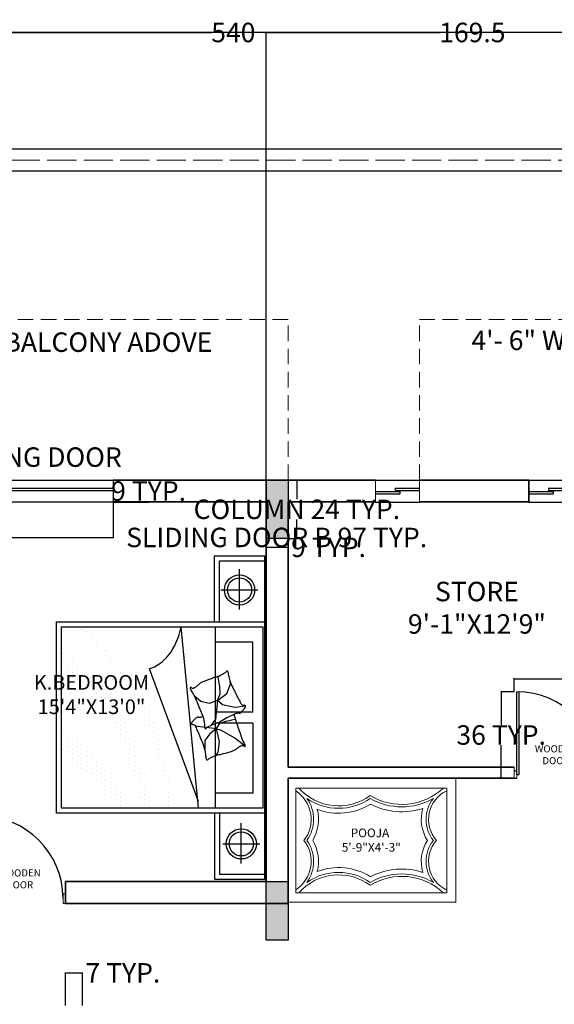
# Model space of a CAD drawing. Units: inches. Extents: x -48 to 50072, y 0 to 21068.
# Tile 55 of 75: x 196 to 415, y 819 to 1224. Entities that reach past the tile are written whole.
import ezdxf

# ---------------------------------------------------------------- set-up
doc = ezdxf.new("R2010")
doc.units = ezdxf.units.IN
doc.header["$MEASUREMENT"] = 0
doc.linetypes.add('ACAD_ISO02W100', pattern=[15, 12, -3])
doc.linetypes.add('HIDDEN', pattern=[9.525, 6.35, -3.175])
for name, color, linetype, lineweight in [('A-ANNO-DIMS', 2, 'Continuous', 18), ('A-ANNO-TEXT', 7, 'Continuous', 18), ('A-AREA-IDEN', 7, 'Continuous', 18), ('A-COLS', 1, 'Continuous', 35), ('A-DOOR', 4, 'Continuous', 18), ('A-FLOR-CASE', 9, 'Continuous', 18), ('A-FLOR-OVHD', 8, 'HIDDEN', 13), ('A-GLAZ', 4, 'Continuous', 18), ('A-WALL', 7, 'Continuous', 35), ('C-PROP', 7, 'Continuous', 25), ('C-PROP-REF', 32, 'ACAD_ISO02W100', 13), ('FURNITURE', 44, 'Continuous', 18)]:
    doc.layers.add(name, color=color, linetype=linetype, lineweight=lineweight)
doc.layers.add('Layer3', color=176, linetype='Continuous')
doc.styles.get("Standard").update_dxf_attribs({"font": 'arial.ttf'})
doc.dimstyles.get("Standard").update_dxf_attribs({"dimtxt": 8, "dimasz": 0.18, "dimexe": 0.18, "dimexo": 0.0625, "dimgap": 0.09, "dimtad": 0, "dimtih": 1, "dimtoh": 1, "dimdec": 1, "dimzin": 0, "dimdsep": 46, "dimlunit": 4, "dimtxsty": 'Standard', "dimblk": 'ARCHTICK', "dimcen": 0.09, "dimadec": 0, "dimazin": 0, "dimtfac": 1, "dimtdec": 1, "dimtofl": 0, "dimtmove": 0, "dimatfit": 3, "dimldrblk": 'ARCHTICK', "dimfxl": 1, "dimtolj": 1, "dimtzin": 0, "dimarcsym": 0})

# ---------------------------------------------------------------- blocks, each defined once
blk = doc.blocks.new('BKUHJKKUG')
at = {"layer": 'Defpoints'}
for p, q in [((179.52, 862.77), (179.52, 896.77)), ((180.52, 862.77), (180.52, 896.76)), ((179.52, 862.77), (180.52, 862.77))]:
    blk.add_line(p, q, dxfattribs=at)
blk.add_arc((179.52, 862.77), 34, 0, 90, dxfattribs=at)
at = {"insert": (190.84, 874.8), "char_height": 2.9183, "attachment_point": 1}
blk.add_mtext_dynamic_manual_height_columns('\\pxqc;WOODEN ^JDOOR', width=9.6242, gutter_width=14.59, heights=[0], dxfattribs=at)
blk = doc.blocks.new('sliding')
blk.add_line((137.02, 1025.77), (137.02, 1034.77))
at = {"layer": 'Defpoints'}
for p, q in [((234.12, 1034.77), (234.12, 1025.77)), ((137.02, 1030.07), (187.57, 1030.07)), ((137.02, 1029.07), (187.57, 1029.07)), ((183.57, 1031.47), (234.12, 1031.47)), ((183.57, 1031.47), (183.57, 1030.47)), ((183.57, 1030.47), (234.12, 1030.47)), ((187.57, 1030.07), (187.57, 1029.07))]:
    blk.add_line(p, q, dxfattribs=at)
at = {"layer": 'Layer3'}
for p, q in [((137.02, 1034.77), (234.12, 1034.77)), ((234.12, 1025.77), (137.02, 1025.77))]:
    blk.add_line(p, q, dxfattribs=at)
blk = doc.blocks.new('bnniku')
at = {"layer": 'Defpoints'}
h = blk.add_hatch(color=256, dxfattribs=at)
h.dxf.hatch_style = 1
h.paths.add_polyline_path([(767.55, 1114.04), (758.55, 1114.04), (758.55, 1090.04), (767.55, 1090.04)])
for p, q in [((758.55, 1114.04), (767.55, 1114.04)), ((758.55, 1090.04), (758.55, 1114.04)), ((767.55, 1114.04), (767.55, 1090.04)), ((767.55, 1090.04), (758.55, 1090.04))]:
    blk.add_line(p, q, dxfattribs=at)
blk = doc.blocks.new('jyugcli')
for p, q in [((342.02, 1025.77), (342.02, 1034.77)), ((360.02, 1025.77), (360.02, 1034.77))]:
    blk.add_line(p, q)
at = {"layer": 'Defpoints'}
for p, q in [((342.02, 1030.07), (352.02, 1030.07)), ((342.02, 1029.07), (352.02, 1029.07)), ((350.02, 1031.47), (360.02, 1031.47)), ((350.02, 1031.47), (350.02, 1030.47)), ((350.02, 1030.47), (360.02, 1030.47)), ((352.02, 1030.07), (352.02, 1029.07))]:
    blk.add_line(p, q, dxfattribs=at)
at = {"layer": 'Layer3'}
for p, q in [((342.02, 1034.77), (360.02, 1034.77)), ((342.02, 1025.77), (360.02, 1025.77))]:
    blk.add_line(p, q, dxfattribs=at)
blk = doc.blocks.new('yfhjudru')
for p, q in [((399.02, 912.27), (399.02, 916.77)), ((400.02, 912.27), (400.02, 915.27)), ((434.02, 912.27), (434.02, 915.27)), ((435.02, 912.27), (435.02, 916.77))]:
    blk.add_line(p, q)
at = {"layer": 'Defpoints'}
for p, q in [((399.02, 915.27), (400.02, 915.27)), ((434.02, 915.27), (435.02, 915.27)), ((399.02, 912.27), (400.02, 912.27)), ((434.02, 912.27), (435.02, 912.27))]:
    blk.add_line(p, q, dxfattribs=at)
blk.add_blockref('BKUHJKKUG', (220.5, 51), dxfattribs=at)
blk = doc.blocks.new('nhrygfdu7yu')
at = {"layer": 'Defpoints'}
for p, q in [((1019.17, 828.61), (845.97, 828.61)), ((845.97, 801.61), (845.97, 828.61)), ((848.67, 804.31), (848.67, 828.61)), ((881.27, 716.83), (881.27, 828.61)), ((983.87, 828.61), (983.87, 716.83)), ((1016.47, 804.31), (1016.47, 828.61)), ((1019.17, 801.61), (1019.17, 828.61)), ((864.18, 805.04), (864.18, 824.84)), ((884.03, 719.53), (884.03, 827.53)), ((884.03, 827.53), (981.17, 827.53)), ((981.17, 827.53), (981.17, 719.53)), ((1000.24, 805.98), (1000.24, 825.78)), ((892.12, 822.13), (892.12, 801.97)), ((929.67, 822.13), (892.12, 822.13)), ((926.47, 818.07), (927.21, 812.5)), ((929.67, 822.13), (929.67, 801.78)), ((935.52, 822.13), (935.52, 801.78)), ((935.52, 822.13), (973.07, 822.13)), ((947.88, 818.06), (943.61, 812.45)), ((973.07, 822.13), (973.07, 801.97)), ((874.65, 814.99), (853.09, 814.99)), ((927.21, 812.5), (925.82, 805.91)), ((934.43, 807.75), (933.36, 812.55)), ((1010.72, 815.93), (989.15, 815.93)), ((914.58, 810.18), (913.28, 809.99)), ((919.69, 808.14), (914.58, 810.18)), ((923.4, 803.12), (919.69, 808.14)), ((935.49, 804.66), (934.43, 807.75)), ((943.61, 812.45), (939.55, 805.41)), ((881.07, 804.31), (848.67, 804.31)), ((881.07, 804.31), (881.07, 804.31)), ((884.06, 801.97), (981.18, 801.97)), ((910.77, 803.49), (910.59, 803.15)), ((916.07, 804.42), (910.77, 803.49)), ((919.78, 804.61), (916.07, 804.42)), ((923.4, 803.12), (919.78, 804.61)), ((925.82, 805.91), (923.4, 803.12)), ((923.4, 803.12), (925.08, 798.67)), ((923.4, 803.12), (933.44, 802.1)), ((933.44, 802.1), (936.13, 800.15)), ((935.45, 803.17), (936.69, 800.13)), ((938.59, 802.42), (935.49, 804.66)), ((938.59, 802.42), (937.95, 797.34)), ((939.55, 805.41), (938.59, 802.42)), ((938.59, 802.42), (945.53, 804.13)), ((938.59, 802.42), (941.26, 799.01)), ((945.53, 804.13), (951.08, 803.38)), ((951.08, 803.38), (953.02, 802.3)), ((984.07, 804.31), (1016.47, 804.31)), ((984.07, 804.31), (984.07, 804.31)), ((881.07, 801.61), (845.97, 801.61)), ((925.08, 798.67), (923.96, 794.21)), ((936.13, 800.15), (936.78, 799.69)), ((936.69, 800.13), (937.65, 797.78)), ((941.26, 799.01), (944.78, 796.45)), ((984.07, 801.61), (1019.17, 801.61)), ((981.13, 793.06), (883.98, 783.7)), ((906.36, 766.47), (977.44, 792.73)), ((923.96, 794.21), (921.07, 790.83)), ((937.86, 796.54), (937.22, 791.44)), ((944.78, 796.45), (949.8, 796.45)), ((962.27, 776.79), (962.27, 776.79)), ((964.84, 776.79), (964.84, 776.79)), ((967.41, 776.79), (967.41, 776.79)), ((969.98, 776.79), (969.98, 776.79)), ((972.55, 776.79), (972.55, 776.79)), ((975.13, 776.79), (975.13, 776.79)), ((976.41, 779.36), (976.41, 779.36)), ((977.7, 776.79), (977.7, 776.79)), ((978.98, 779.36), (978.98, 779.36)), ((980.27, 776.79), (980.27, 776.79)), ((941.69, 771.64), (941.69, 771.64)), ((944.27, 771.64), (944.27, 771.64)), ((946.84, 771.64), (946.84, 771.64)), ((949.41, 771.64), (949.41, 771.64)), ((950.69, 774.21), (950.69, 774.21)), ((951.98, 771.64), (951.98, 771.64)), ((953.27, 774.21), (953.27, 774.21)), ((954.55, 771.64), (954.55, 771.64)), ((955.84, 774.21), (955.84, 774.21)), ((958.41, 774.21), (958.41, 774.21)), ((960.98, 774.21), (960.98, 774.21)), ((963.55, 774.21), (963.55, 774.21)), ((966.13, 774.21), (966.13, 774.21)), ((968.7, 774.21), (968.7, 774.21)), ((928.83, 766.5), (928.83, 766.5)), ((931.41, 766.5), (931.41, 766.5)), ((933.98, 766.5), (933.98, 766.5)), ((935.26, 769.07), (935.26, 769.07)), ((936.55, 766.5), (936.55, 766.5)), ((937.84, 769.07), (937.84, 769.07)), ((940.41, 769.07), (940.41, 769.07)), ((942.98, 769.07), (942.98, 769.07)), ((975.13, 766.5), (975.13, 766.5)), ((977.7, 766.5), (977.7, 766.5)), ((980.27, 766.5), (980.27, 766.5)), ((921.12, 761.35), (921.12, 761.35)), ((923.69, 761.35), (923.69, 761.35)), ((924.98, 763.93), (924.98, 763.93)), ((927.55, 763.93), (927.55, 763.93)), ((930.12, 763.93), (930.12, 763.93)), ((954.55, 761.35), (954.55, 761.35)), ((957.12, 761.35), (957.12, 761.35)), ((959.7, 761.35), (959.7, 761.35)), ((962.27, 761.35), (962.27, 761.35)), ((963.55, 763.93), (963.55, 763.93)), ((964.84, 761.35), (964.84, 761.35)), ((966.13, 763.93), (966.13, 763.93)), ((967.41, 761.35), (967.41, 761.35)), ((968.7, 763.93), (968.7, 763.93)), ((969.98, 761.35), (969.98, 761.35)), ((971.27, 763.93), (971.27, 763.93)), ((972.55, 761.35), (972.55, 761.35)), ((973.84, 763.93), (973.84, 763.93)), ((975.13, 761.35), (975.13, 761.35)), ((976.41, 763.93), (976.41, 763.93)), ((978.98, 763.93), (978.98, 763.93)), ((913.4, 756.21), (913.4, 756.21)), ((915.98, 756.21), (915.98, 756.21)), ((917.26, 758.78), (917.26, 758.78)), ((919.83, 758.78), (919.83, 758.78)), ((941.69, 756.21), (941.69, 756.21)), ((944.27, 756.21), (944.27, 756.21)), ((945.55, 758.78), (945.55, 758.78)), ((946.84, 756.21), (946.84, 756.21)), ((948.12, 758.78), (948.12, 758.78)), ((949.41, 756.21), (949.41, 756.21)), ((950.69, 758.78), (950.69, 758.78)), ((951.98, 756.21), (951.98, 756.21)), ((953.27, 758.78), (953.27, 758.78)), ((954.55, 756.21), (954.55, 756.21)), ((955.84, 758.78), (955.84, 758.78)), ((957.12, 756.21), (957.12, 756.21)), ((958.41, 758.78), (958.41, 758.78)), ((960.98, 758.78), (960.98, 758.78)), ((963.55, 758.78), (963.55, 758.78)), ((980.27, 756.21), (980.27, 756.21)), ((905.69, 751.07), (905.69, 751.07)), ((908.26, 751.07), (908.26, 751.07)), ((909.55, 753.64), (909.55, 753.64)), ((912.12, 753.64), (912.12, 753.64)), ((931.41, 751.07), (931.41, 751.07)), ((933.98, 751.07), (933.98, 751.07)), ((935.26, 753.64), (935.26, 753.64)), ((936.55, 751.07), (936.55, 751.07)), ((937.84, 753.64), (937.84, 753.64)), ((939.12, 751.07), (939.12, 751.07)), ((940.41, 753.64), (940.41, 753.64)), ((941.69, 751.07), (941.69, 751.07)), ((942.98, 753.64), (942.98, 753.64)), ((944.27, 751.07), (944.27, 751.07)), ((945.55, 753.64), (945.55, 753.64)), ((948.12, 753.64), (948.12, 753.64)), ((969.98, 751.07), (969.98, 751.07)), ((972.55, 751.07), (972.55, 751.07)), ((975.13, 751.07), (975.13, 751.07)), ((976.41, 753.64), (976.41, 753.64)), ((977.7, 751.07), (977.7, 751.07)), ((978.98, 753.64), (978.98, 753.64)), ((980.27, 751.07), (980.27, 751.07)), ((900.55, 745.92), (900.55, 745.92)), ((903.12, 745.92), (903.12, 745.92)), ((904.4, 748.5), (904.4, 748.5)), ((923.69, 745.92), (923.69, 745.92)), ((926.26, 745.92), (926.26, 745.92)), ((927.55, 748.5), (927.55, 748.5)), ((928.83, 745.92), (928.83, 745.92)), ((930.12, 748.5), (930.12, 748.5)), ((931.41, 745.92), (931.41, 745.92)), ((932.69, 748.5), (932.69, 748.5)), ((933.98, 745.92), (933.98, 745.92)), ((935.26, 748.5), (935.26, 748.5)), ((937.84, 748.5), (937.84, 748.5)), ((940.41, 748.5), (940.41, 748.5)), ((962.27, 745.92), (962.27, 745.92)), ((964.84, 745.92), (964.84, 745.92)), ((966.13, 748.5), (966.13, 748.5)), ((967.41, 745.92), (967.41, 745.92)), ((968.7, 748.5), (968.7, 748.5)), ((969.98, 745.92), (969.98, 745.92)), ((971.27, 748.5), (971.27, 748.5)), ((972.55, 745.92), (972.55, 745.92)), ((973.84, 748.5), (973.84, 748.5)), ((975.13, 745.92), (975.13, 745.92)), ((976.41, 748.5), (976.41, 748.5)), ((977.7, 745.92), (977.7, 745.92)), ((978.98, 748.5), (978.98, 748.5)), ((895.4, 740.78), (895.4, 740.78)), ((896.69, 743.35), (896.69, 743.35)), ((899.26, 743.35), (899.26, 743.35)), ((915.98, 740.78), (915.98, 740.78)), ((918.55, 740.78), (918.55, 740.78)), ((919.83, 743.35), (919.83, 743.35)), ((921.12, 740.78), (921.12, 740.78)), ((922.41, 743.35), (922.41, 743.35)), ((923.69, 740.78), (923.69, 740.78)), ((924.98, 743.35), (924.98, 743.35)), ((926.26, 740.78), (926.26, 740.78)), ((927.55, 743.35), (927.55, 743.35)), ((928.83, 740.78), (928.83, 740.78)), ((930.12, 743.35), (930.12, 743.35)), ((932.69, 743.35), (932.69, 743.35)), ((957.12, 740.78), (957.12, 740.78)), ((959.7, 740.78), (959.7, 740.78)), ((960.98, 743.35), (960.98, 743.35)), ((962.27, 740.78), (962.27, 740.78)), ((963.55, 743.35), (963.55, 743.35)), ((964.84, 740.78), (964.84, 740.78)), ((966.13, 743.35), (966.13, 743.35)), ((967.41, 740.78), (967.41, 740.78)), ((968.7, 743.35), (968.7, 743.35)), ((969.98, 740.78), (969.98, 740.78)), ((971.27, 743.35), (971.27, 743.35)), ((973.84, 743.35), (973.84, 743.35)), ((887.69, 735.64), (887.69, 735.64)), ((890.26, 735.64), (890.26, 735.64)), ((891.54, 738.21), (891.54, 738.21)), ((894.12, 738.21), (894.12, 738.21)), ((910.83, 735.64), (910.83, 735.64)), ((913.4, 735.64), (913.4, 735.64)), ((914.69, 738.21), (914.69, 738.21)), ((915.98, 735.64), (915.98, 735.64)), ((917.26, 738.21), (917.26, 738.21)), ((918.55, 735.64), (918.55, 735.64)), ((919.83, 738.21), (919.83, 738.21)), ((921.12, 735.64), (921.12, 735.64)), ((922.41, 738.21), (922.41, 738.21)), ((924.98, 738.21), (924.98, 738.21)), ((951.98, 735.64), (951.98, 735.64)), ((954.55, 735.64), (954.55, 735.64)), ((955.84, 738.21), (955.84, 738.21)), ((957.12, 735.64), (957.12, 735.64)), ((958.41, 738.21), (958.41, 738.21)), ((959.7, 735.64), (959.7, 735.64)), ((960.98, 738.21), (960.98, 738.21)), ((962.27, 735.64), (962.27, 735.64)), ((963.55, 738.21), (963.55, 738.21)), ((964.84, 735.64), (964.84, 735.64)), ((966.13, 738.21), (966.13, 738.21)), ((885.12, 730.49), (885.12, 730.49)), ((886.4, 733.07), (886.4, 733.07)), ((888.97, 733.07), (888.97, 733.07)), ((905.69, 730.49), (905.69, 730.49)), ((908.26, 730.49), (908.26, 730.49)), ((909.55, 733.07), (909.55, 733.07)), ((910.83, 730.49), (910.83, 730.49)), ((912.12, 733.07), (912.12, 733.07)), ((913.4, 730.49), (913.4, 730.49)), ((914.69, 733.07), (914.69, 733.07)), ((915.98, 730.49), (915.98, 730.49)), ((917.26, 733.07), (917.26, 733.07)), ((919.83, 733.07), (919.83, 733.07)), ((946.84, 730.49), (946.84, 730.49)), ((949.41, 730.49), (949.41, 730.49)), ((950.69, 733.07), (950.69, 733.07)), ((951.98, 730.49), (951.98, 730.49)), ((953.27, 733.07), (953.27, 733.07)), ((954.55, 730.49), (954.55, 730.49)), ((955.84, 733.07), (955.84, 733.07)), ((957.12, 730.49), (957.12, 730.49)), ((958.41, 733.07), (958.41, 733.07)), ((959.7, 730.49), (959.7, 730.49)), ((960.98, 733.07), (960.98, 733.07)), ((900.55, 725.35), (900.55, 725.35)), ((903.12, 725.35), (903.12, 725.35)), ((904.4, 727.92), (904.4, 727.92)), ((905.69, 725.35), (905.69, 725.35)), ((906.97, 727.92), (906.97, 727.92)), ((908.26, 725.35), (908.26, 725.35)), ((909.55, 727.92), (909.55, 727.92)), ((910.83, 725.35), (910.83, 725.35)), ((912.12, 727.92), (912.12, 727.92)), ((944.27, 725.35), (944.27, 725.35)), ((945.55, 727.92), (945.55, 727.92)), ((946.84, 725.35), (946.84, 725.35)), ((948.12, 727.92), (948.12, 727.92)), ((949.41, 725.35), (949.41, 725.35)), ((950.69, 727.92), (950.69, 727.92)), ((951.98, 725.35), (951.98, 725.35)), ((953.27, 727.92), (953.27, 727.92)), ((954.55, 725.35), (954.55, 725.35)), ((955.84, 727.92), (955.84, 727.92)), ((958.41, 727.92), (958.41, 727.92)), ((981.17, 719.53), (884.03, 719.53)), ((895.4, 720.21), (895.4, 720.21)), ((897.97, 720.21), (897.97, 720.21)), ((899.26, 722.78), (899.26, 722.78)), ((900.55, 720.21), (900.55, 720.21)), ((901.83, 722.78), (901.83, 722.78)), ((903.12, 720.21), (903.12, 720.21)), ((904.4, 722.78), (904.4, 722.78)), ((905.69, 720.21), (905.69, 720.21)), ((906.97, 722.78), (906.97, 722.78)), ((939.12, 720.21), (939.12, 720.21)), ((941.69, 720.21), (941.69, 720.21)), ((942.98, 722.78), (942.98, 722.78)), ((944.27, 720.21), (944.27, 720.21)), ((945.55, 722.78), (945.55, 722.78)), ((946.84, 720.21), (946.84, 720.21)), ((948.12, 722.78), (948.12, 722.78)), ((949.41, 720.21), (949.41, 720.21)), ((950.69, 722.78), (950.69, 722.78)), ((951.98, 720.21), (951.98, 720.21)), ((953.27, 722.78), (953.27, 722.78)), ((983.87, 716.83), (881.27, 716.83))]:
    blk.add_line(p, q, dxfattribs=at)
for centre, radius in [((864.18, 814.99), 8.1), ((1000.24, 815.93), 8.1), ((864.18, 814.99), 6.48), ((1000.24, 815.93), 6.48)]:
    blk.add_circle(centre, radius, dxfattribs=at)
for centre, radius, start, end in [((926.67, 817.58), 0.687, 51.1864, 183.2455), ((924.75, 815.18), 3.76, 45.8726, 51.1864), ((929.07, 819.63), 2.44, 225.8726, 232.4713), ((948.22, 814.9), 3.25, 110.3452, 128.5854), ((947.75, 816.16), 1.9, 86.0516, 110.3452), ((947.87, 817.82), 0.239, 13.2808, 86.0516), ((947.77, 817.8), 0.34, 306.5792, 13.2808), ((771.78, 1091.44), 315.27, 297.4921, 297.8482), ((1072.97, 521.35), 329.5, 117.4999, 117.8482), ((971.1, 717.04), 108.88, 116.4147, 117.4999), ((848.26, 964.34), 167.25, 296.4147, 297.2902), ((924.05, 817.43), 1.94, 297.2902, 3.2455), ((940.16, 834.08), 20.66, 232.4713, 233.7837), ((906.88, 788.64), 35.67, 52.7849, 53.7837), ((921.35, 807.68), 11.75, 46.4776, 52.7849), ((926.56, 813.17), 4.18, 35.8936, 46.4776), ((928.96, 814.91), 1.22, 351.9508, 35.8936), ((932.62, 814.39), 2.47, 171.9508, 202.4162), ((980.52, 834.15), 54.29, 202.4162, 205.0529), ((883.03, 974.91), 169.83, 286.6085, 289.0836), ((848.62, 1074.38), 275.09, 289.0836, 290.1287), ((927.73, 858.54), 45.2, 290.1287, 292.7069), ((943.53, 820.78), 4.28, 292.7069, 308.5854), ((951.77, 816.3), 4.17, 169.5926, 177.2714), ((948.44, 816.46), 0.826, 177.2714, 194.5709), ((949.69, 816.78), 2.12, 194.5709, 206.8179), ((948.43, 816.91), 0.765, 126.5792, 169.5926), ((964.76, 824.4), 19.01, 206.8179, 210.9056), ((957.44, 820.02), 10.47, 210.9056, 219.7005), ((946.01, 810.53), 4.37, 26.0735, 39.7005), ((908.02, 808.45), 0.313, 121.6917, 179.0386), ((908.61, 808.44), 0.905, 179.0386, 229.4914), ((909.3, 806.38), 2.75, 103.0402, 121.6917), ((905.38, 804.66), 4.08, 26.3332, 49.4914), ((909.41, 805.91), 3.23, 86.6119, 103.0402), ((909.8, 812.53), 3.4, 266.6119, 282.6252), ((905.47, 831.87), 23.22, 282.6252, 290.7486), ((901.77, 841.65), 33.68, 290.7486, 297.4921), ((929.77, 818.2), 6.29, 280.7366, 286.6085), ((1013.86, 849.73), 91.09, 205.0529, 207.0884), ((1008.01, 846.74), 84.52, 207.0884, 209.936), ((940.41, 807.79), 10.61, 17.8396, 26.0735), ((847.55, 777.91), 108.16, 15.2625, 17.8396), ((780.21, 742.7), 143.74, 25.1732, 26.3332), ((901.51, 799.71), 9.71, 20.7081, 25.1732), ((883.04, 792.73), 29.45, 18.2369, 20.7081), ((995.54, 829.8), 89, 198.2369, 199.6584), ((924.73, 798.79), 11.57, 22.2355, 29.936), ((866.04, 782.95), 89, 13.841, 15.2625), ((981.05, 811.29), 29.45, 193.841, 196.3122), ((962.1, 805.74), 9.71, 196.3122, 200.7773), ((1087.42, 853.29), 143.74, 200.7773, 201.9373), ((1013.59, 836.25), 108.16, 199.6584, 202.2355), ((938.8, 798.25), 1.24, 202.2355, 252.8133), ((938.36, 796.82), 0.252, 289.3799, 72.8133), ((955.69, 773.98), 23.22, 98.2293, 106.3527), ((952.85, 793.6), 3.4, 82.216, 98.2293), ((953.75, 800.17), 3.23, 262.216, 278.6443), ((957.87, 801.11), 4.08, 201.9373, 225.0955), ((953.82, 799.69), 2.75, 278.6443, 297.2959), ((954.35, 797.58), 0.905, 354.6428, 45.0955), ((954.94, 797.53), 0.313, 297.2959, 354.6428), ((923.29, 799.33), 10.61, 202.2355, 210.4694), ((917.92, 796.17), 4.37, 210.4694, 224.0964), ((907.26, 785.84), 10.47, 35.3015, 44.0964), ((900.29, 780.91), 19.01, 31.2138, 35.3015), ((1035.25, 540.56), 275.09, 113.4795, 114.5246), ((993.31, 637.11), 169.83, 111.0043, 113.4795), ((880.68, 777.46), 54.29, 18.0203, 19.3448), ((929.96, 793.49), 2.47, 347.5549, 18.0203), ((933.57, 792.7), 1.22, 167.5549, 211.4977), ((934.7, 789.77), 6.29, 98.1216, 111.0043), ((936.09, 794.24), 4.18, 211.4977, 222.0817), ((941.71, 799.32), 11.75, 222.0817, 228.389), ((934.31, 792.46), 3.58, 85.4882, 98.1216), ((934.9, 799.87), 3.85, 265.4882, 277.6784), ((934.12, 805.65), 9.69, 277.6784, 284.8807), ((938.27, 789.81), 1.94, 112.8944, 178.8496), ((939.32, 786.09), 10.56, 97.9822, 104.8807), ((1002.58, 637.52), 167.25, 112.0188, 112.8944), ((938.1, 794.73), 1.83, 85.7407, 97.9822), ((938.28, 797.05), 0.497, 265.7407, 289.3799), ((899.06, 893.51), 108.88, 292.0188, 293.104), ((812.48, 1096.43), 329.5, 293.104, 293.4523), ((1069.09, 504.93), 315.27, 113.0962, 113.4523), ((958.63, 763.95), 33.68, 106.3527, 113.0962), ((916.73, 788.79), 0.34, 130.9751, 197.6767), ((916.63, 788.76), 0.239, 197.6767, 270.4475), ((916, 789.63), 0.765, 310.9751, 353.9885), ((914.73, 789.66), 2.12, 18.9668, 31.2138), ((916.62, 790.42), 1.9, 270.4475, 294.7411), ((915.96, 790.08), 0.826, 1.6673, 18.9668), ((912.62, 789.98), 4.17, 353.9885, 1.6673), ((916.05, 791.65), 3.25, 294.7411, 312.9813), ((921.18, 786.14), 4.28, 117.1028, 132.9813), ((939.83, 749.71), 45.2, 114.5246, 117.1028), ((957.59, 817.2), 35.67, 228.389, 229.3878), ((920.93, 774.44), 20.66, 48.0754, 49.3878), ((933.1, 787.99), 2.44, 41.4767, 48.0754), ((937.75, 792.1), 3.76, 221.4767, 226.7905), ((935.64, 789.86), 0.687, 226.7905, 358.8496)]:
    blk.add_arc(centre, radius, start, end, dxfattribs=at)
blk.add_ellipse((874.1, 762.91), major_axis=(32.71, 0), ratio=0.667085, start_param=0.16392, end_param=1.263761, dxfattribs=at)
blk = doc.blocks.new('_ArchTick')
at = {"color": 0, "linetype": 'ByBlock', "const_width": 0.15}
blk.add_lwpolyline([(-0.5, -0.5), (0.5, 0.5)], dxfattribs=at)
blk = doc.blocks.new('*D48')
at = {"layer": 'A-ANNO-DIMS', "color": 0, "lineweight": -2, "transparency": 16777216}
for p, q in [((306.08, 1034.77), (309.8, 1034.77)), ((309.62, 1034.77), (309.62, 1027)), ((309.62, 1010.77), (309.62, 1018.55)), ((306.08, 1010.77), (309.8, 1010.77))]:
    blk.add_line(p, q, dxfattribs=at)
at = {"layer": 'Defpoints', "color": 0, "transparency": 16777216}
for p in [(306.02, 1034.77), (309.62, 1034.77), (306.02, 1010.77)]:
    blk.add_point(p, dxfattribs=at)
at = {"layer": 'A-ANNO-DIMS', "color": 0, "lineweight": -2, "transparency": 16777216, "xscale": 0.18, "yscale": 0.18, "zscale": 0.18}
for p, rotation in [((309.62, 1034.77), 90), ((309.62, 1010.77), 270)]:
    blk.add_blockref('_ArchTick', p, dxfattribs=dict(at, rotation=rotation))
at = {"layer": 'A-ANNO-DIMS', "color": 0, "transparency": 16777216, "insert": (309.62, 1022.77), "char_height": 8, "attachment_point": 5}
blk.add_mtext('\\A1;COLUMN 24 TYP.', dxfattribs=at)
blk = doc.blocks.new('*D49')
at = {"layer": 'A-ANNO-DIMS', "color": 0, "lineweight": -2, "transparency": 16777216}
for p, q in [((297.02, 1010.71), (297.02, 1006.99)), ((306.02, 1010.71), (306.02, 1006.99)), ((297.02, 1007.17), (306.02, 1007.17)), ((306.02, 1007.17), (306.2, 1007.17))]:
    blk.add_line(p, q, dxfattribs=at)
at = {"layer": 'Defpoints', "color": 0, "transparency": 16777216}
for p in [(297.02, 1010.77), (306.02, 1010.77), (306.02, 1007.17)]:
    blk.add_point(p, dxfattribs=at)
at = {"layer": 'A-ANNO-DIMS', "color": 0, "lineweight": -2, "transparency": 16777216, "xscale": 0.18, "yscale": 0.18, "zscale": 0.18, "rotation": 180}
blk.add_blockref('_ArchTick', (297.02, 1007.17), dxfattribs=at)
at = {"layer": 'A-ANNO-DIMS', "color": 0, "lineweight": -2, "transparency": 16777216, "xscale": 0.18, "yscale": 0.18, "zscale": 0.18}
blk.add_blockref('_ArchTick', (306.02, 1007.17), dxfattribs=at)
at = {"layer": 'A-ANNO-DIMS', "color": 0, "transparency": 16777216, "insert": (322.65, 1007.17), "char_height": 8, "attachment_point": 5}
blk.add_mtext('\\A1;9 TYP.', dxfattribs=at)
blk = doc.blocks.new('*D62')
at = {"layer": 'A-ANNO-DIMS', "color": 0, "lineweight": -2, "transparency": 16777216}
for p, q in [((137.02, 1025.71), (137.02, 1011.03)), ((234.12, 1025.71), (234.12, 1011.03)), ((137.02, 1011.21), (234.12, 1011.21)), ((234.12, 1011.21), (234.3, 1011.21))]:
    blk.add_line(p, q, dxfattribs=at)
at = {"layer": 'Defpoints', "color": 0, "transparency": 16777216}
for p in [(137.02, 1025.77), (234.12, 1025.77), (234.12, 1011.21)]:
    blk.add_point(p, dxfattribs=at)
at = {"layer": 'A-ANNO-DIMS', "color": 0, "lineweight": -2, "transparency": 16777216, "xscale": 0.18, "yscale": 0.18, "zscale": 0.18, "rotation": 180}
blk.add_blockref('_ArchTick', (137.02, 1011.21), dxfattribs=at)
at = {"layer": 'A-ANNO-DIMS', "color": 0, "lineweight": -2, "transparency": 16777216, "xscale": 0.18, "yscale": 0.18, "zscale": 0.18}
blk.add_blockref('_ArchTick', (234.12, 1011.21), dxfattribs=at)
at = {"layer": 'A-ANNO-DIMS', "color": 0, "transparency": 16777216, "insert": (301.34, 1011.21), "char_height": 8, "attachment_point": 5}
blk.add_mtext('\\A1;SLIDING DOOR B 97 TYP.', dxfattribs=at)
blk = doc.blocks.new('*D63')
at = {"layer": 'A-ANNO-DIMS', "color": 0, "lineweight": -2, "transparency": 16777216}
for p, q in [((234.18, 1034.77), (248.86, 1034.77)), ((248.68, 1034.77), (248.68, 1034.45)), ((234.18, 1025.77), (248.86, 1025.77)), ((248.68, 1025.77), (248.68, 1026.1))]:
    blk.add_line(p, q, dxfattribs=at)
at = {"layer": 'Defpoints', "color": 0, "transparency": 16777216}
for p in [(234.12, 1034.77), (248.68, 1034.77), (234.12, 1025.77)]:
    blk.add_point(p, dxfattribs=at)
at = {"layer": 'A-ANNO-DIMS', "color": 0, "lineweight": -2, "transparency": 16777216, "xscale": 0.18, "yscale": 0.18, "zscale": 0.18}
for p, rotation in [((248.68, 1034.77), 90), ((248.68, 1025.77), 270)]:
    blk.add_blockref('_ArchTick', p, dxfattribs=dict(at, rotation=rotation))
at = {"layer": 'A-ANNO-DIMS', "color": 0, "transparency": 16777216, "insert": (248.68, 1030.27), "char_height": 8, "attachment_point": 5}
blk.add_mtext('\\A1;9 TYP.', dxfattribs=at)
blk = doc.blocks.new('*D64')
at = {"layer": 'A-ANNO-DIMS', "color": 0, "lineweight": -2, "transparency": 16777216}
for p, q in [((399.02, 947.84), (399.02, 953.35)), ((399.02, 953.17), (435.02, 953.17)), ((435.02, 947.84), (435.02, 953.35)), ((435.02, 953.17), (435.2, 953.17))]:
    blk.add_line(p, q, dxfattribs=at)
at = {"layer": 'Defpoints', "color": 0, "transparency": 16777216}
for p in [(435.02, 953.17), (399.02, 947.77), (435.02, 947.77)]:
    blk.add_point(p, dxfattribs=at)
at = {"layer": 'A-ANNO-DIMS', "color": 0, "lineweight": -2, "transparency": 16777216, "xscale": 0.18, "yscale": 0.18, "zscale": 0.18, "rotation": 180}
blk.add_blockref('_ArchTick', (399.02, 953.17), dxfattribs=at)
at = {"layer": 'A-ANNO-DIMS', "color": 0, "lineweight": -2, "transparency": 16777216, "xscale": 0.18, "yscale": 0.18, "zscale": 0.18}
blk.add_blockref('_ArchTick', (435.02, 953.17), dxfattribs=at)
at = {"layer": 'A-ANNO-DIMS', "color": 0, "transparency": 16777216, "insert": (491.8, 953.17), "char_height": 8, "attachment_point": 5}
blk.add_mtext('\\A1;ROOM DOOR 36 TYP.', dxfattribs=at)
blk = doc.blocks.new('*D65')
at = {"layer": 'A-ANNO-DIMS', "color": 0, "lineweight": -2, "transparency": 16777216}
for p, q in [((398.95, 947.77), (393.44, 947.77)), ((393.62, 947.77), (393.62, 934.2)), ((393.62, 912.27), (393.62, 925.85)), ((398.95, 912.27), (393.44, 912.27))]:
    blk.add_line(p, q, dxfattribs=at)
at = {"layer": 'Defpoints', "color": 0, "transparency": 16777216}
for p in [(393.62, 947.77), (399.02, 947.77), (399.02, 912.27)]:
    blk.add_point(p, dxfattribs=at)
at = {"layer": 'A-ANNO-DIMS', "color": 0, "lineweight": -2, "transparency": 16777216, "xscale": 0.18, "yscale": 0.18, "zscale": 0.18}
for p, rotation in [((393.62, 947.77), 90), ((393.62, 912.27), 270)]:
    blk.add_blockref('_ArchTick', p, dxfattribs=dict(at, rotation=rotation))
at = {"layer": 'A-ANNO-DIMS', "color": 0, "transparency": 16777216, "insert": (393.62, 930.02), "char_height": 8, "attachment_point": 5}
blk.add_mtext('\\A1;36 TYP.', dxfattribs=at)
blk = doc.blocks.new('*D101')
at = {"layer": 'A-ANNO-DIMS', "color": 0, "lineweight": -2, "transparency": 16777216}
for p, q in [((214.52, 818.84), (214.52, 832.45)), ((214.52, 832.27), (221.52, 832.27)), ((221.52, 818.84), (221.52, 832.45)), ((221.52, 832.27), (221.7, 832.27))]:
    blk.add_line(p, q, dxfattribs=at)
at = {"layer": 'Defpoints', "color": 0, "transparency": 16777216}
for p in [(221.52, 832.27), (214.52, 818.77), (221.52, 818.77)]:
    blk.add_point(p, dxfattribs=at)
at = {"layer": 'A-ANNO-DIMS', "color": 0, "lineweight": -2, "transparency": 16777216, "xscale": 0.18, "yscale": 0.18, "zscale": 0.18, "rotation": 180}
blk.add_blockref('_ArchTick', (214.52, 832.27), dxfattribs=at)
at = {"layer": 'A-ANNO-DIMS', "color": 0, "lineweight": -2, "transparency": 16777216, "xscale": 0.18, "yscale": 0.18, "zscale": 0.18}
blk.add_blockref('_ArchTick', (221.52, 832.27), dxfattribs=at)
at = {"layer": 'A-ANNO-DIMS', "color": 0, "transparency": 16777216, "insert": (238.12, 832.27), "char_height": 8, "attachment_point": 5}
blk.add_mtext('\\A1;7 TYP.', dxfattribs=at)
blk = doc.blocks.new('*D112')
at = {"layer": 'A-ANNO-DIMS', "color": 0, "lineweight": -2, "transparency": 16777216}
for p, q in [((13.52, 1170.84), (13.52, 1218.9)), ((13.52, 1218.72), (274.6, 1218.72)), ((553.52, 1218.72), (292.43, 1218.72)), ((553.52, 1170.84), (553.52, 1218.9))]:
    blk.add_line(p, q, dxfattribs=at)
at = {"layer": 'Defpoints', "color": 0, "transparency": 16777216}
for p in [(553.52, 1218.72), (13.52, 1170.77), (553.52, 1170.77)]:
    blk.add_point(p, dxfattribs=at)
at = {"layer": 'A-ANNO-DIMS', "color": 0, "lineweight": -2, "transparency": 16777216, "xscale": 0.18, "yscale": 0.18, "zscale": 0.18, "rotation": 180}
blk.add_blockref('_ArchTick', (13.52, 1218.72), dxfattribs=at)
at = {"layer": 'A-ANNO-DIMS', "color": 0, "lineweight": -2, "transparency": 16777216, "xscale": 0.18, "yscale": 0.18, "zscale": 0.18}
blk.add_blockref('_ArchTick', (553.52, 1218.72), dxfattribs=at)
at = {"layer": 'A-ANNO-DIMS', "color": 0, "transparency": 16777216, "insert": (283.52, 1218.72), "char_height": 8, "attachment_point": 5}
blk.add_mtext('\\A1;540', dxfattribs=at)
blk = doc.blocks.new('*D123')
at = {"layer": 'A-ANNO-DIMS', "color": 0, "lineweight": -2, "transparency": 16777216}
for p, q in [((18.02, 1034.84), (18.02, 1218.9)), ((18.02, 1218.72), (148.51, 1218.72)), ((297.02, 1218.72), (166.52, 1218.72)), ((297.02, 1034.84), (297.02, 1218.9))]:
    blk.add_line(p, q, dxfattribs=at)
at = {"layer": 'Defpoints', "color": 0, "transparency": 16777216}
for p in [(297.02, 1218.72), (18.02, 1034.77), (297.02, 1034.77)]:
    blk.add_point(p, dxfattribs=at)
at = {"layer": 'A-ANNO-DIMS', "color": 0, "lineweight": -2, "transparency": 16777216, "xscale": 0.18, "yscale": 0.18, "zscale": 0.18, "rotation": 180}
blk.add_blockref('_ArchTick', (18.02, 1218.72), dxfattribs=at)
at = {"layer": 'A-ANNO-DIMS', "color": 0, "lineweight": -2, "transparency": 16777216, "xscale": 0.18, "yscale": 0.18, "zscale": 0.18}
blk.add_blockref('_ArchTick', (297.02, 1218.72), dxfattribs=at)
at = {"layer": 'A-ANNO-DIMS', "color": 0, "transparency": 16777216, "insert": (157.52, 1218.72), "char_height": 8, "attachment_point": 5}
blk.add_mtext('\\A1;279', dxfattribs=at)
blk = doc.blocks.new('*D124')
at = {"layer": 'A-ANNO-DIMS', "color": 0, "lineweight": -2, "transparency": 16777216}
for p, q in [((297.02, 1034.84), (297.02, 1218.9)), ((297.02, 1218.72), (368.53, 1218.72)), ((466.52, 1218.72), (395.01, 1218.72)), ((466.52, 1034.84), (466.52, 1218.9))]:
    blk.add_line(p, q, dxfattribs=at)
at = {"layer": 'Defpoints', "color": 0, "transparency": 16777216}
for p in [(466.52, 1218.72), (297.02, 1034.77), (466.52, 1034.77)]:
    blk.add_point(p, dxfattribs=at)
at = {"layer": 'A-ANNO-DIMS', "color": 0, "lineweight": -2, "transparency": 16777216, "xscale": 0.18, "yscale": 0.18, "zscale": 0.18, "rotation": 180}
blk.add_blockref('_ArchTick', (297.02, 1218.72), dxfattribs=at)
at = {"layer": 'A-ANNO-DIMS', "color": 0, "lineweight": -2, "transparency": 16777216, "xscale": 0.18, "yscale": 0.18, "zscale": 0.18}
blk.add_blockref('_ArchTick', (466.52, 1218.72), dxfattribs=at)
at = {"layer": 'A-ANNO-DIMS', "color": 0, "transparency": 16777216, "insert": (381.77, 1218.72), "char_height": 8, "attachment_point": 5}
blk.add_mtext('\\A1;169.5', dxfattribs=at)

msp = doc.modelspace()

# ---------------------------------------------------------------- linework, layer by layer
at = {"layer": 'A-DOOR'}
for p, q in [((213.517, 864.775), (213.517, 860.775)), ((213.517, 864.775), (214.517, 864.775)), ((213.517, 860.775), (214.517, 860.775))]:
    msp.add_line(p, q, dxfattribs=at)
at = {"layer": 'A-FLOR-CASE'}
for q in [(375.017, 912.275), (306.017, 861.275)]:
    msp.add_line((375.017, 861.275), q, dxfattribs=at)
msp.add_lwpolyline([(309.173, 908.23), (371.276, 908.23), (371.276, 865.208), (309.173, 865.208)], close=True, dxfattribs=at)
for points in [[(365.735, 886.719, 0.3438536), (365.735, 869.475, 0.2669418), (339.763, 869.475, 0.3134227), (313.791, 869.475, 0.3166326), (313.791, 886.719, 0.3166326), (313.791, 903.963, 0.3134227), (339.763, 903.963, 0.2669418), (365.735, 903.963, 0.3438536)], [(363.289, 886.719, 0.2170719), (361.425, 873.567, 0.2005492), (339.859, 871.806, 0.2339356), (318.004, 873.938, 0.1975179), (316.169, 886.719, 0.1975179), (318.004, 899.5, 0.2339356), (339.859, 901.632, 0.2005492), (361.425, 899.871, 0.2170719)]]:
    msp.add_lwpolyline(points, format="xyb", close=True, dxfattribs=at)
for centre, radius, start, end in [((301.541, 895.341), 13.98, 321.9221, 56.90879), ((326.777, 922.644), 21.752, 221.5027, 306.48505), ((352.749, 926.553), 25.057, 238.6445, 313.00906), ((376.79, 895.341), 13.019, 115.05718, 221.47015), ((301.541, 878.097), 13.98, 303.09121, 38.0779), ((376.79, 878.097), 13.019, 138.52985, 244.94282), ((326.777, 850.794), 21.752, 53.51495, 138.4973), ((352.749, 846.885), 25.057, 46.99094, 121.3555)]:
    msp.add_arc(centre, radius, start, end, dxfattribs=at)
at = {"layer": 'A-FLOR-OVHD'}
for p, q in [((306.017, 1100.775), (105.517, 1100.775)), ((306.017, 1034.775), (306.017, 1100.775)), ((360.017, 1034.775), (360.017, 1100.775)), ((360.017, 1100.775), (544.517, 1100.775))]:
    msp.add_line(p, q, dxfattribs=at)
at = {"layer": 'A-WALL'}
for p, q in [((342.017, 1034.775), (234.116, 1034.775)), ((297.017, 869.775), (297.017, 1034.775)), ((405.017, 1034.775), (360.017, 1034.775)), ((405.017, 1025.775), (405.017, 1034.775)), ((297.017, 1025.775), (234.116, 1025.775)), ((306.017, 916.775), (306.017, 1025.775)), ((342.017, 1025.775), (306.017, 1025.775)), ((405.017, 1025.775), (360.017, 1025.775)), ((399.017, 916.775), (306.017, 916.775)), ((306.017, 860.775), (306.017, 912.275)), ((399.017, 912.275), (306.017, 912.275)), ((297.017, 869.775), (214.517, 869.775)), ((214.517, 869.775), (214.517, 860.775)), ((306.017, 860.775), (214.517, 860.775))]:
    msp.add_line(p, q, dxfattribs=at)
at = {"layer": 'C-PROP'}
for p, q in [((553.517, 1170.775), (13.517, 1170.775)), ((544.517, 1161.775), (22.517, 1161.775))]:
    msp.add_line(p, q, dxfattribs=at)
at = {"layer": 'C-PROP-REF'}
msp.add_line((549.017, 1166.275), (18.017, 1166.275), dxfattribs=at)

# ---------------------------------------------------------------- block references
at = {"layer": 'A-COLS'}
for p in [(-461.534, -79.262), (-461.534, -244.262)]:
    msp.add_blockref('bnniku', p, dxfattribs=at)
at = {"layer": 'A-DOOR'}
for name in ['sliding', 'yfhjudru', 'BKUHJKKUG']:
    msp.add_blockref(name, (0, 0), dxfattribs=at)
at = {"layer": 'A-GLAZ'}
for p in [(0, 0), (63, 0)]:
    msp.add_blockref('jyugcli', p, dxfattribs=at)
at = {"layer": 'FURNITURE', "xscale": 0.7669307891904348, "yscale": 0.7669307891904348, "zscale": 0.7669307891904348, "rotation": 270}
msp.add_blockref('nhrygfdu7yu', (-338.974, 1652.402), dxfattribs=at)

# ---------------------------------------------------------------- texts
at = {"layer": 'A-ANNO-TEXT', "char_height": 8, "attachment_point": 1}
for s, width, insert in [('4\'- 6" WILD BALCONY ADOVE ', 220.65422, (381.401, 1096.216)), ('5\'- 6" WILD BALCONY ADOVE ', 220.65422, (131.359, 1095.463)), ('UPVC SLIDING DOOR ', 126.59735, (132.36, 1048.223))]:
    msp.add_mtext_dynamic_manual_height_columns(s, width=width, gutter_width=40, heights=[0], dxfattribs=dict(at, insert=insert))
at = {"layer": 'A-AREA-IDEN', "attachment_point": 1}
for s, width, gutter_width, insert, char_height in [('\\pxqc;STORE ^J9\'-1"X12\'9"', 250.42359, 40, (258.441, 992.986), 8), ('\\pxqc;K.BEDROOM^J15\'4"X13\'0"', 75.10877, 30, (187.667, 954.642), 6), ('\\pxqc;POOJA^J 5\'-9"X4\'-3"', 54.37376, 17.82, (312.5, 891.579), 3.56406)]:
    msp.add_mtext_dynamic_manual_height_columns(s, width=width, gutter_width=gutter_width, heights=[0], dxfattribs=dict(at, insert=insert, char_height=char_height))

# ---------------------------------------------------------------- dimensions: what is measured, and where the dimension line sits
at = {"layer": 'A-ANNO-DIMS'}
for base, p1, p2, override, picture, middle in [((553.517, 1218.725), (13.517, 1170.775), (553.517, 1170.775), {"dimdec": 0, "dimlfac": 1, "dimrnd": 0, "dimzin": 0, "dimdsep": 46, "dimlunit": 2}, '*D112', (283.517, 1218.725)), ((297.017, 1218.725), (18.017, 1034.775), (297.017, 1034.775), {"dimdec": 0, "dimlfac": 1, "dimrnd": 0, "dimzin": 0, "dimdsep": 46, "dimlunit": 2}, '*D123', (157.517, 1218.725)), ((466.517, 1218.725), (297.017, 1034.775), (466.517, 1034.775), {"dimdec": 1, "dimlfac": 1, "dimrnd": 0, "dimzin": 0, "dimdsep": 46, "dimlunit": 2}, '*D124', (381.767, 1218.725))]:
    dim = msp.add_linear_dim(base=base, p1=p1, p2=p2, dimstyle='Standard', override=override, dxfattribs=at)
    dim.commit()
    dim.dimension.update_dxf_attribs({"geometry": picture, "text_midpoint": middle})
for base, p1, p2, text, picture, middle in [((234.116, 1011.21), (137.017, 1025.775), (234.116, 1025.775), 'SLIDING DOOR B <> TYP.', '*D62', (301.343, 1011.21)), ((306.017, 1007.175), (297.017, 1010.775), (306.017, 1010.775), '<> TYP.', '*D49', (322.65, 1007.175)), ((435.017, 953.175), (399.017, 947.775), (435.017, 947.775), 'ROOM DOOR <> TYP.', '*D64', (491.803, 953.175)), ((221.517, 832.275), (214.517, 818.775), (221.517, 818.775), '<> TYP.', '*D101', (238.118, 832.275))]:
    dim = msp.add_linear_dim(base=base, p1=p1, p2=p2, text=text, dimstyle='Standard', override={"dimdec": 0, "dimlfac": 1, "dimrnd": 0, "dimzin": 0, "dimdsep": 46, "dimlunit": 2}, dxfattribs=at)
    dim.commit()
    dim.dimension.update_dxf_attribs({"geometry": picture, "text_midpoint": middle})
for base, p1, p2, text, picture, middle in [((248.681, 1034.775), (234.116, 1025.775), (234.116, 1034.775), '<> TYP.', '*D63', (248.681, 1030.275)), ((309.617, 1034.775), (306.017, 1010.775), (306.017, 1034.775), 'COLUMN <> TYP.', '*D48', (309.617, 1022.775)), ((393.617152656, 947.774790015), (399.017152656, 912.274790015), (399.017152656, 947.774790015), '<> TYP.', '*D65', (393.617152656, 930.024790015))]:
    dim = msp.add_linear_dim(base=base, p1=p1, p2=p2, angle=90, text=text, dimstyle='Standard', override={"dimdec": 0, "dimlfac": 1, "dimrnd": 0, "dimzin": 0, "dimdsep": 46, "dimlunit": 2}, dxfattribs=at)
    dim.commit()
    dim.dimension.update_dxf_attribs({"geometry": picture, "text_midpoint": middle})

doc.saveas('drawing.dxf')
